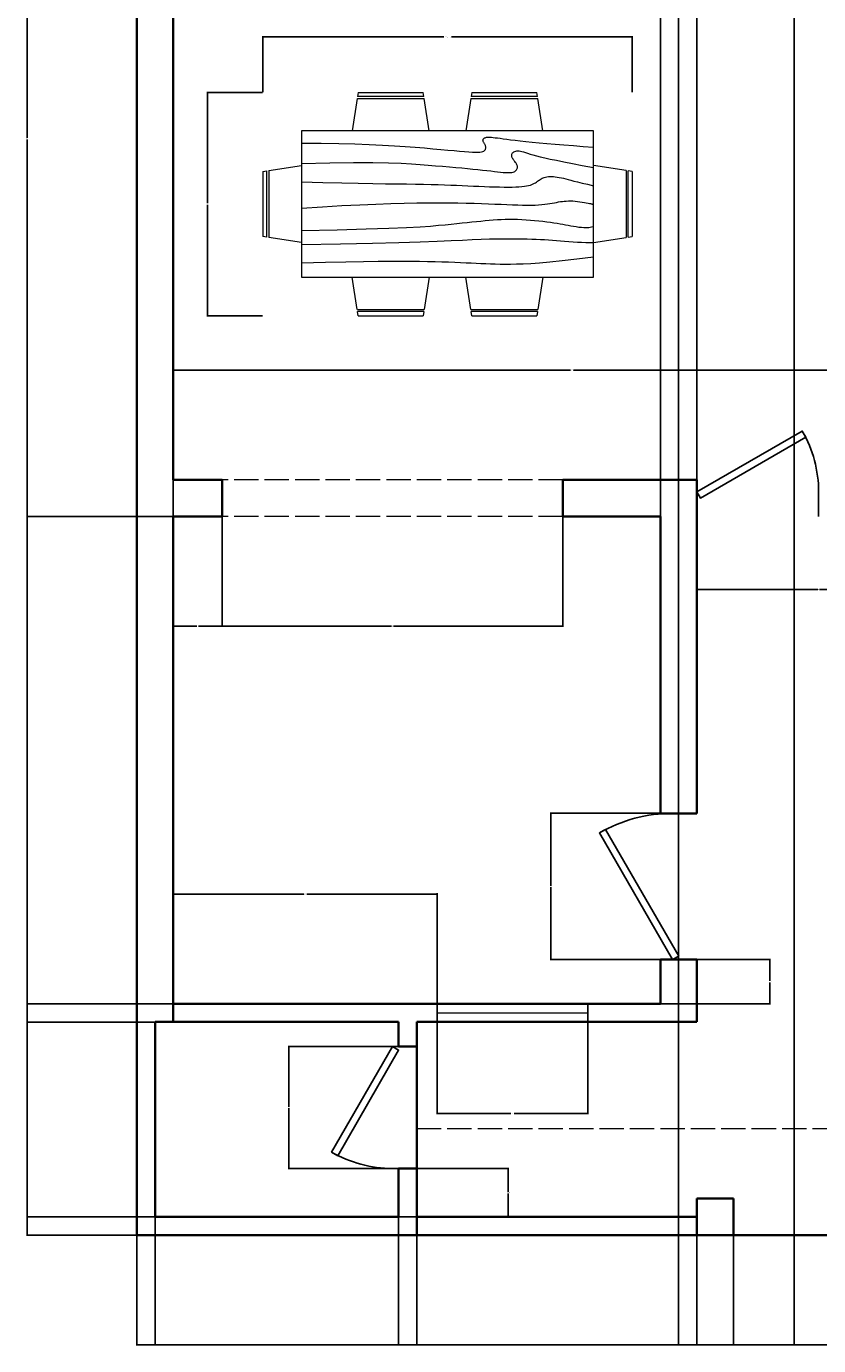
# Model space of a CAD drawing. Units: inches. Extents: x 2599 to 2953, y 557 to 1152.
# Tile 1 of 7: x 2599 to 2794, y 557 to 882. Entities that reach past the tile are written whole.
import ezdxf

# ---------------------------------------------------------------- set-up
doc = ezdxf.new("R2010")
doc.units = ezdxf.units.IN
doc.linetypes.add('ACAD_ISO02W100', pattern=[15, 12, -3])
for name, color, linetype, lineweight in [('A-ANNO-DIMS', 2, 'Continuous', 18), ('A-COLS', 7, 'Continuous', 35), ('A-DOOR', 4, 'Continuous', 25), ('A-FURN', 8, 'Continuous', 18), ('A-GLAZ', 4, 'Continuous', 18), ('A-WALL', 7, 'Continuous', 35), ('A-WALL-OVHD', 8, 'ACAD_ISO02W100', 18)]:
    doc.layers.add(name, color=color, linetype=linetype, lineweight=lineweight)
doc.styles.get("Standard").update_dxf_attribs({"font": 'arial.ttf'})
doc.dimstyles.get("Standard").update_dxf_attribs({"dimtxt": 0.18, "dimasz": 0.18, "dimexe": 0.18, "dimexo": 0.0625, "dimgap": 0.09, "dimtad": 0, "dimtih": 1, "dimtoh": 1, "dimdec": 4, "dimzin": 0, "dimdsep": 46, "dimtxsty": 'Standard', "dimcen": 0.09, "dimadec": 0, "dimazin": 0, "dimtfac": 1, "dimtdec": 4, "dimtofl": 0, "dimtmove": 0, "dimatfit": 3, "dimfxl": 1, "dimtolj": 1, "dimtzin": 0, "dimarcsym": 0})

# ---------------------------------------------------------------- blocks, each defined once
blk = doc.blocks.new('*U3')
for p, q in [((-30, 0), (-30, -6)), ((0, 0), (0, -6))]:
    blk.add_line(p, q)
blk.add_lwpolyline([(0, 0), (-25.98, 15), (-26.86, 13.48), (-0.88, -1.52)], close=True)
blk.add_arc((0, 0), 30, 150, 180)
blk = doc.blocks.new('*U4')
for p, q in [((0, 0), (0, -6)), ((36, 0), (36, -6))]:
    blk.add_line(p, q)
blk.add_lwpolyline([(0, 0), (31.18, 18), (32.05, 16.48), (0.87, -1.52)], close=True)
blk.add_arc((0, 0), 36, 0, 30)
blk = doc.blocks.new('*U5')
for p, q in [((0, 0), (0, -6)), ((30, 0), (30, -6))]:
    blk.add_line(p, q)
blk.add_lwpolyline([(0, 0), (25.98, 15), (26.86, 13.48), (0.87, -1.52)], close=True)
blk.add_arc((0, 0), 30, 0, 30)
blk = doc.blocks.new('Dining Set - 36 x 72 in.')
for p, q in [((-22.2343, 26.00059), (-23.4847, 17.99762)), ((-22.2304, 26), (-5.7608, 26)), ((-22, 27.5), (-22.1562, 26.50042)), ((-5.8416, 26.5), (-22.1534, 26.5)), ((-22, 27.5), (-6, 27.5)), ((-5.8437, 26.49966), (-6, 27.5)), ((-4.5152, 17.99762), (-5.7655, 25.99926)), ((5.7657, 26.00059), (4.5153, 17.99762)), ((5.7696, 26), (22.2392, 26)), ((6, 27.5), (5.8438, 26.50042)), ((22.1584, 26.5), (5.8466, 26.5)), ((6, 27.5), (22, 27.5)), ((22.1563, 26.49966), (22, 27.5)), ((23.4848, 17.99762), (22.2345, 25.99926)), ((36, 18), (-36, 18)), ((-36, 18), (-36, -18)), ((36, -18), (36, 18)), ((-45.5, 8), (-44.5004, 8.15617)), ((-45.5, 8), (-45.5, -8)), ((-44.5, -8.15843), (-44.5, 8.15338)), ((-44.0006, 8.23428), (-35.9976, 9.48474)), ((-44, 8.23041), (-44, -8.23915)), ((44.0006, 8.23428), (35.9976, 9.48474)), ((44, 8.23041), (44, -8.23915)), ((44.5, -8.15843), (44.5, 8.15338)), ((45.5, 8), (44.5005, 8.15617)), ((45.5, 8), (45.5, -8)), ((-44.4997, -8.15631), (-45.5, -8)), ((-35.9976, -9.48476), (-43.9993, -8.2345)), ((35.9976, -9.48476), (43.9993, -8.2345)), ((44.4997, -8.15631), (45.5, -8)), ((-36, -18), (36, -18)), ((-22.2343, -26.0006), (-23.4847, -17.99762)), ((-4.5152, -17.99762), (-5.7655, -25.99928)), ((5.7657, -26.0006), (4.5153, -17.99762)), ((23.4848, -17.99762), (22.2345, -25.99928)), ((-22.2304, -26), (-5.7608, -26)), ((-22, -27.5), (-22.1562, -26.50044)), ((-5.8416, -26.5), (-22.1534, -26.5)), ((-22, -27.5), (-6, -27.5)), ((-5.8437, -26.49967), (-6, -27.5)), ((5.7696, -26), (22.2392, -26)), ((6, -27.5), (5.8438, -26.50044)), ((22.1584, -26.5), (5.8466, -26.5)), ((6, -27.5), (22, -27.5)), ((22.1563, -26.49967), (22, -27.5))]:
    blk.add_line(p, q)
for points in [[(-36, 15), (-31.1772, 14.97754), (-26.8079, 14.91406), (-22.8538, 14.81543), (-19.276, 14.6875), (-16.0362, 14.53613), (-13.0957, 14.36718), (-10.4159, 14.18652), (-7.9583, 14), (-5.6904, 13.81315), (-3.6035, 13.63021), (-1.6954, 13.45508), (0.0365, 13.29166), (1.5945, 13.14388), (2.9811, 13.01562), (4.1988, 12.9108), (5.25, 12.83333), (6.1393, 12.78613), (6.8802, 12.76823), (7.4883, 12.77767), (7.9792, 12.8125), (8.3685, 12.87077), (8.6719, 12.95052), (8.9049, 13.0498), (9.0833, 13.16666), (9.2205, 13.29899), (9.3216, 13.44401), (9.3895, 13.59879), (9.4271, 13.76041), (9.4373, 13.92594), (9.4232, 14.09245), (9.3875, 14.257), (9.3333, 14.41666), (9.2638, 14.56917), (9.1836, 14.71484), (9.0975, 14.85465), (9.0104, 14.98958), (8.9272, 15.1206), (8.8529, 15.2487), (8.7922, 15.37483), (8.75, 15.5), (8.7305, 15.62467), (8.7344, 15.74739), (8.7617, 15.86621), (8.8125, 15.97916), (8.8867, 16.08431), (8.9844, 16.17968), (9.1055, 16.26334), (9.25, 16.33333), (9.4189, 16.38802), (9.6172, 16.42708), (9.8506, 16.45052), (10.125, 16.45833), (10.4463, 16.45052), (10.8203, 16.42708), (11.2529, 16.38802), (11.75, 16.33333), (12.3184, 16.26318), (12.9694, 16.17838), (13.7151, 16.07991), (14.5677, 15.96875), (15.5395, 15.84586), (16.6426, 15.71224), (17.8893, 15.56884), (19.2917, 15.41666), (20.859, 15.25667), (22.5879, 15.08984), (24.4721, 14.91715), (26.5052, 14.73958), (28.6809, 14.5581), (30.9929, 14.3737), (33.4347, 14.18733), (36, 14)], [(-36, 10), (-28.9766, 10.14274), (-23.1725, 10.20442), (-18.4241, 10.19775), (-14.5677, 10.13541), (-11.4399, 10.03011), (-8.877, 9.89453), (-6.7154, 9.74137), (-4.7917, 9.58333), (-2.9698, 9.43082), (-1.2246, 9.28515), (0.4415, 9.14534), (2.026, 9.01041), (3.5266, 8.87939), (4.9408, 8.7513), (6.266, 8.62516), (7.5, 8.5), (8.6411, 8.37549), (9.6914, 8.2539), (10.6538, 8.13818), (11.5312, 8.03125), (12.3267, 7.93603), (13.043, 7.85547), (13.6831, 7.79248), (14.25, 7.75), (14.7471, 7.7303), (15.1797, 7.73307), (15.5537, 7.75732), (15.875, 7.80208), (16.1494, 7.86637), (16.3828, 7.94922), (16.5811, 8.04964), (16.75, 8.16666), (16.8944, 8.29915), (17.0143, 8.44531), (17.1089, 8.60319), (17.1771, 8.77083), (17.218, 8.94629), (17.2305, 9.1276), (17.2137, 9.31282), (17.1667, 9.5), (17.0895, 9.6875), (16.987, 9.875), (16.8649, 10.0625), (16.7292, 10.25), (16.5856, 10.4375), (16.4401, 10.625), (16.2985, 10.8125), (16.1667, 11), (16.05, 11.18733), (15.9518, 11.3737), (15.8752, 11.5581), (15.8229, 11.73958), (15.798, 11.91715), (15.8034, 12.08984), (15.842, 12.25667), (15.9167, 12.41666), (16.0295, 12.56836), (16.1784, 12.70833), (16.3605, 12.83268), (16.5729, 12.9375), (16.8127, 13.01888), (17.0768, 13.07291), (17.3625, 13.0957), (17.6667, 13.08333), (17.9894, 13.03312), (18.3418, 12.94726), (18.7382, 12.82918), (19.1927, 12.68229), (19.7195, 12.51001), (20.3327, 12.31575), (21.0465, 12.10294), (21.875, 11.875), (22.8357, 11.63354), (23.959, 11.37304), (25.2786, 11.08618), (26.8282, 10.76562), (28.6414, 10.40405), (30.752, 9.99414), (33.1936, 9.52856), (36, 9)], [(-36, 5.5), (-30.7157, 5.3348), (-26.069, 5.20963), (-21.9946, 5.11767), (-18.4271, 5.05208), (-15.3009, 5.00602), (-12.5508, 4.97265), (-10.1112, 4.94515), (-7.9167, 4.91666), (-5.909, 4.88167), (-4.0586, 4.83984), (-2.3429, 4.79215), (-0.7396, 4.73958), (0.7739, 4.6831), (2.22, 4.6237), (3.6213, 4.56233), (5, 4.5), (6.373, 4.43782), (7.7344, 4.3776), (9.0723, 4.32129), (10.375, 4.27083), (11.6309, 4.22819), (12.8281, 4.19531), (13.9551, 4.17415), (15, 4.16666), (15.954, 4.17448), (16.819, 4.19791), (17.6001, 4.23698), (18.3021, 4.29166), (18.9299, 4.36198), (19.4883, 4.44791), (19.9823, 4.54948), (20.4167, 4.66666), (20.7969, 4.79899), (21.1302, 4.94401), (21.4245, 5.09879), (21.6875, 5.26041), (21.9271, 5.42594), (22.1511, 5.59245), (22.3672, 5.757), (22.5834, 5.91666), (22.8065, 6.06868), (23.0404, 6.21093), (23.2879, 6.34147), (23.5521, 6.45833), (23.8358, 6.55957), (24.142, 6.64323), (24.4735, 6.70735), (24.8334, 6.75), (25.2235, 6.76969), (25.642, 6.76692), (26.0858, 6.74267), (26.5521, 6.69791), (27.0379, 6.63362), (27.5404, 6.55078), (28.0565, 6.45036), (28.5834, 6.33333), (29.1242, 6.19987), (29.7071, 6.04687), (30.3661, 5.87044), (31.1354, 5.66666), (32.0493, 5.43164), (33.142, 5.16146), (34.4475, 4.85221), (36, 4.5)], [(-36, -1), (-30.7915, -0.6591), (-26.0195, -0.38216), (-21.6519, -0.16284), (-17.6563, 0.00521), (-14.0005, 0.12833), (-10.6523, 0.21289), (-7.5796, 0.26522), (-4.75, 0.29166), (-2.134, 0.29793), (0.2878, 0.28711), (2.5317, 0.26163), (4.6146, 0.22396), (6.5529, 0.17651), (8.3633, 0.12174), (10.0623, 0.06209), (11.6667, 0), (13.1899, -0.06201), (14.6341, -0.1211), (15.9982, -0.17432), (17.2813, -0.21875), (18.4823, -0.25147), (19.6003, -0.26953), (20.6343, -0.27002), (21.5834, -0.25), (22.4481, -0.20768), (23.2357, -0.14584), (23.9549, -0.06836), (24.6146, 0.02083), (25.2235, 0.11784), (25.7904, 0.21875), (26.3241, 0.31966), (26.8334, 0.41666), (27.3265, 0.50618), (27.8099, 0.58593), (28.2894, 0.65397), (28.7709, 0.70833), (29.2601, 0.74707), (29.763, 0.76823), (30.2855, 0.76985), (30.8334, 0.75), (31.4088, 0.70784), (31.9994, 0.64713), (32.589, 0.57275), (33.1615, 0.48958), (33.7008, 0.4025), (34.1908, 0.3164), (34.6153, 0.23616), (34.9584, 0.16666), (35.2099, 0.11165), (35.3848, 0.07031), (35.504, 0.04069), (35.5886, 0.02083), (35.6594, 0.00879), (35.7377, 0.0026), (35.8442, 0.00032), (36, 0)], [(-36, -6.5), (-27.1843, -6.31267), (-20.084, -6.1263), (-14.469, -5.9419), (-10.1094, -5.76042), (-6.7752, -5.58285), (-4.2363, -5.41016), (-2.2629, -5.24333), (-0.625, -5.08334), (0.8708, -4.93099), (2.2715, -4.78646), (3.5872, -4.64974), (4.8281, -4.52084), (6.0046, -4.39974), (7.127, -4.28646), (8.2053, -4.18099), (9.25, -4.08334), (10.2705, -3.99382), (11.2734, -3.91407), (12.2647, -3.84603), (13.25, -3.79167), (14.2354, -3.75293), (15.2266, -3.73177), (16.2295, -3.73015), (17.25, -3.75), (18.2912, -3.79248), (19.3451, -3.85547), (20.4009, -3.93604), (21.4479, -4.03125), (22.4754, -4.13819), (23.4727, -4.25391), (24.4289, -4.37549), (25.3334, -4.5), (26.1785, -4.62492), (26.9694, -4.74935), (27.7145, -4.87281), (28.4219, -4.99479), (29.1, -5.11483), (29.7572, -5.23242), (30.4016, -5.34709), (31.0417, -5.45834), (31.6837, -5.56437), (32.3262, -5.65821), (32.9658, -5.73153), (33.599, -5.77604), (34.2224, -5.78345), (34.8327, -5.74545), (35.4264, -5.65373), (36, -5.5)], [(-36, -10), (-26.4022, -9.81299), (-18.4675, -9.62891), (-11.9839, -9.45069), (-6.7396, -9.28125), (-2.5226, -9.12354), (0.8789, -8.98047), (3.6769, -8.85498), (6.0833, -8.75), (8.2767, -8.66765), (10.3021, -8.60677), (12.1712, -8.56543), (13.8958, -8.54167), (15.4876, -8.53353), (16.9583, -8.53907), (18.3197, -8.55632), (19.5834, -8.58334), (20.7616, -8.61841), (21.8685, -8.66081), (22.9188, -8.71004), (23.9271, -8.76563), (24.9081, -8.82707), (25.8763, -8.89388), (26.8465, -8.96558), (27.8334, -9.04167), (28.8474, -9.12118), (29.8828, -9.20117), (30.93, -9.27824), (31.9792, -9.34896), (33.0205, -9.40991), (34.0443, -9.45768), (35.0407, -9.48885), (36, -9.5)], [(-36, -14.5), (-30.0881, -14.33513), (-25.0332, -14.21224), (-20.7312, -14.12647), (-17.0781, -14.07292), (-13.97, -14.04671), (-11.3027, -14.04297), (-8.9724, -14.05681), (-6.875, -14.08334), (-4.9224, -14.11833), (-3.0905, -14.16016), (-1.3709, -14.20785), (0.2448, -14.26042), (1.7647, -14.3169), (3.1973, -14.3763), (4.5507, -14.43767), (5.8333, -14.5), (7.0554, -14.5621), (8.235, -14.62175), (9.3922, -14.67652), (10.5469, -14.72396), (11.7192, -14.76164), (12.929, -14.78711), (14.1965, -14.79794), (15.5417, -14.79167), (16.9933, -14.76424), (18.6152, -14.70508), (20.4804, -14.60197), (22.6615, -14.44271), (25.2312, -14.21509), (28.2624, -13.9069), (31.8277, -13.50594), (36, -13)]]:
    blk.add_lwpolyline(points)
blk = doc.blocks.new('*D17')
at = {"layer": 'A-ANNO-DIMS', "color": 0, "lineweight": -2, "transparency": 16777216}
for p, q in [((2656.99, 865.8), (2656.99, 879.57)), ((2657.17, 879.39), (2701.54, 879.39)), ((2747.81, 879.39), (2703.44, 879.39)), ((2747.99, 865.8), (2747.99, 879.57))]:
    blk.add_line(p, q, dxfattribs=at)
at = {"layer": 'A-ANNO-DIMS', "color": 0, "transparency": 16777216}
for points in [[(2657.17, 879.42), (2657.17, 879.36), (2656.99, 879.39)], [(2747.81, 879.42), (2747.81, 879.36), (2747.99, 879.39)]]:
    blk.add_solid(points, dxfattribs=at)
at = {"layer": 'Defpoints', "color": 0, "transparency": 16777216}
for p in [(2747.99, 879.39), (2656.99, 865.74), (2747.99, 865.74)]:
    blk.add_point(p, dxfattribs=at)
at = {"layer": 'A-ANNO-DIMS', "color": 0, "transparency": 16777216, "insert": (2702.49, 879.39), "char_height": 0.18, "attachment_point": 5}
blk.add_mtext('\\A1;DINING SET 91', dxfattribs=at)
blk = doc.blocks.new('*D18')
at = {"layer": 'A-ANNO-DIMS', "color": 0, "lineweight": -2, "transparency": 16777216}
for p, q in [((2656.93, 865.74), (2643.16, 865.74)), ((2643.34, 865.56), (2643.34, 838.42)), ((2643.34, 810.92), (2643.34, 838.06)), ((2656.93, 810.74), (2643.16, 810.74))]:
    blk.add_line(p, q, dxfattribs=at)
at = {"layer": 'A-ANNO-DIMS', "color": 0, "transparency": 16777216}
for points in [[(2643.31, 865.56), (2643.37, 865.56), (2643.34, 865.74)], [(2643.31, 810.92), (2643.37, 810.92), (2643.34, 810.74)]]:
    blk.add_solid(points, dxfattribs=at)
at = {"layer": 'Defpoints', "color": 0, "transparency": 16777216}
for p in [(2643.34, 865.74), (2656.99, 865.74), (2656.99, 810.74)]:
    blk.add_point(p, dxfattribs=at)
at = {"layer": 'A-ANNO-DIMS', "color": 0, "transparency": 16777216, "insert": (2643.34, 838.24), "char_height": 0.18, "attachment_point": 5}
blk.add_mtext('\\A1;55', dxfattribs=at)
blk = doc.blocks.new('*D21')
at = {"layer": 'A-ANNO-DIMS', "color": 0, "lineweight": -2, "transparency": 16777216}
for p, q in [((2625.92, 1124.28), (2625.92, 557.16)), ((2925.92, 584.28), (2925.92, 557.16)), ((2626.1, 557.34), (2775.63, 557.34)), ((2925.74, 557.34), (2776.21, 557.34))]:
    blk.add_line(p, q, dxfattribs=at)
at = {"layer": 'A-ANNO-DIMS', "color": 0, "transparency": 16777216}
for points in [[(2626.1, 557.37), (2626.1, 557.31), (2625.92, 557.34)], [(2925.74, 557.37), (2925.74, 557.31), (2925.92, 557.34)]]:
    blk.add_solid(points, dxfattribs=at)
at = {"layer": 'Defpoints', "color": 0, "transparency": 16777216}
for p in [(2625.92, 1124.34), (2925.92, 584.34), (2925.92, 557.34)]:
    blk.add_point(p, dxfattribs=at)
at = {"layer": 'A-ANNO-DIMS', "color": 0, "transparency": 16777216, "insert": (2775.92, 557.34), "char_height": 0.18, "attachment_point": 5}
blk.add_mtext('\\A1;300', dxfattribs=at)
blk = doc.blocks.new('*D22')
at = {"layer": 'A-ANNO-DIMS', "color": 0, "lineweight": -2, "transparency": 16777216}
for p, q in [((2625.86, 1124.34), (2598.74, 1124.34)), ((2598.92, 1124.16), (2598.92, 854.52)), ((2598.92, 584.52), (2598.92, 854.16)), ((2625.86, 584.34), (2598.74, 584.34))]:
    blk.add_line(p, q, dxfattribs=at)
at = {"layer": 'A-ANNO-DIMS', "color": 0, "transparency": 16777216}
for points in [[(2598.89, 1124.16), (2598.95, 1124.16), (2598.92, 1124.34)], [(2598.89, 584.52), (2598.95, 584.52), (2598.92, 584.34)]]:
    blk.add_solid(points, dxfattribs=at)
at = {"layer": 'Defpoints', "color": 0, "transparency": 16777216}
for p in [(2598.92, 1124.34), (2625.92, 1124.34), (2625.92, 584.34)]:
    blk.add_point(p, dxfattribs=at)
at = {"layer": 'A-ANNO-DIMS', "color": 0, "transparency": 16777216, "insert": (2598.92, 854.34), "char_height": 0.18, "attachment_point": 5}
blk.add_mtext('\\A1;540', dxfattribs=at)
blk = doc.blocks.new('*D23')
at = {"layer": 'A-ANNO-DIMS', "color": 0, "lineweight": -2, "transparency": 16777216}
for p, q in [((2634.92, 770.4), (2634.92, 797.53)), ((2635.1, 797.35), (2732.79, 797.35)), ((2831.24, 797.35), (2733.56, 797.35)), ((2831.42, 770.4), (2831.42, 797.53))]:
    blk.add_line(p, q, dxfattribs=at)
at = {"layer": 'A-ANNO-DIMS', "color": 0, "transparency": 16777216}
for points in [[(2635.1, 797.38), (2635.1, 797.32), (2634.92, 797.35)], [(2831.24, 797.38), (2831.24, 797.32), (2831.42, 797.35)]]:
    blk.add_solid(points, dxfattribs=at)
at = {"layer": 'Defpoints', "color": 0, "transparency": 16777216}
for p in [(2831.42, 797.35), (2634.92, 770.34), (2831.42, 770.34)]:
    blk.add_point(p, dxfattribs=at)
at = {"layer": 'A-ANNO-DIMS', "color": 0, "transparency": 16777216, "insert": (2733.17, 797.35), "char_height": 0.18, "attachment_point": 5}
blk.add_mtext('\\A1;196.5', dxfattribs=at)
blk = doc.blocks.new('*D28')
at = {"layer": 'A-ANNO-DIMS', "color": 0, "lineweight": -2, "transparency": 16777216}
for p, q in [((2763.92, 770.28), (2763.92, 743.16)), ((2823.92, 770.28), (2823.92, 743.16)), ((2764.1, 743.34), (2793.7, 743.34)), ((2823.74, 743.34), (2794.14, 743.34))]:
    blk.add_line(p, q, dxfattribs=at)
at = {"layer": 'A-ANNO-DIMS', "color": 0, "transparency": 16777216}
for points in [[(2764.1, 743.37), (2764.1, 743.31), (2763.92, 743.34)], [(2823.74, 743.37), (2823.74, 743.31), (2823.92, 743.34)]]:
    blk.add_solid(points, dxfattribs=at)
at = {"layer": 'Defpoints', "color": 0, "transparency": 16777216}
for p in [(2763.92, 770.34), (2823.92, 770.34), (2763.92, 743.34)]:
    blk.add_point(p, dxfattribs=at)
at = {"layer": 'A-ANNO-DIMS', "color": 0, "transparency": 16777216, "insert": (2793.92, 743.34), "char_height": 0.18, "attachment_point": 5}
blk.add_mtext('\\A1;60', dxfattribs=at)
blk = doc.blocks.new('*D32')
at = {"layer": 'A-ANNO-DIMS', "color": 0, "lineweight": -2, "transparency": 16777216}
for p, q in [((2630.42, 588.78), (2630.42, 557.16)), ((2690.42, 588.78), (2690.42, 557.16)), ((2630.6, 557.34), (2660.2, 557.34)), ((2690.24, 557.34), (2660.64, 557.34))]:
    blk.add_line(p, q, dxfattribs=at)
at = {"layer": 'A-ANNO-DIMS', "color": 0, "transparency": 16777216}
for points in [[(2630.6, 557.37), (2630.6, 557.31), (2630.42, 557.34)], [(2690.24, 557.37), (2690.24, 557.31), (2690.42, 557.34)]]:
    blk.add_solid(points, dxfattribs=at)
at = {"layer": 'Defpoints', "color": 0, "transparency": 16777216}
for p in [(2630.42, 588.84), (2690.42, 588.84), (2690.42, 557.34)]:
    blk.add_point(p, dxfattribs=at)
at = {"layer": 'A-ANNO-DIMS', "color": 0, "transparency": 16777216, "insert": (2660.42, 557.34), "char_height": 0.18, "attachment_point": 5}
blk.add_mtext('\\A1;60', dxfattribs=at)
blk = doc.blocks.new('*D33')
at = {"layer": 'A-ANNO-DIMS', "color": 0, "lineweight": -2, "transparency": 16777216}
for p, q in [((2630.36, 636.84), (2598.74, 636.84)), ((2598.92, 636.66), (2598.92, 613.02)), ((2598.92, 589.02), (2598.92, 612.66)), ((2630.36, 588.84), (2598.74, 588.84))]:
    blk.add_line(p, q, dxfattribs=at)
at = {"layer": 'A-ANNO-DIMS', "color": 0, "transparency": 16777216}
for points in [[(2598.89, 636.66), (2598.95, 636.66), (2598.92, 636.84)], [(2598.89, 589.02), (2598.95, 589.02), (2598.92, 588.84)]]:
    blk.add_solid(points, dxfattribs=at)
at = {"layer": 'Defpoints', "color": 0, "transparency": 16777216}
for p in [(2598.92, 636.84), (2630.42, 636.84), (2630.42, 588.84)]:
    blk.add_point(p, dxfattribs=at)
at = {"layer": 'A-ANNO-DIMS', "color": 0, "transparency": 16777216, "insert": (2598.92, 612.84), "char_height": 0.18, "attachment_point": 5}
blk.add_mtext('\\A1;48', dxfattribs=at)
blk = doc.blocks.new('*D34')
at = {"layer": 'A-ANNO-DIMS', "color": 0, "lineweight": -2, "transparency": 16777216}
for p, q in [((2694.92, 584.28), (2694.92, 557.16)), ((2763.92, 584.28), (2763.92, 557.16)), ((2695.1, 557.34), (2729.2, 557.34)), ((2763.74, 557.34), (2729.64, 557.34))]:
    blk.add_line(p, q, dxfattribs=at)
at = {"layer": 'A-ANNO-DIMS', "color": 0, "transparency": 16777216}
for points in [[(2695.1, 557.37), (2695.1, 557.31), (2694.92, 557.34)], [(2763.74, 557.37), (2763.74, 557.31), (2763.92, 557.34)]]:
    blk.add_solid(points, dxfattribs=at)
at = {"layer": 'Defpoints', "color": 0, "transparency": 16777216}
for p in [(2694.92, 584.34), (2763.92, 584.34), (2763.92, 557.34)]:
    blk.add_point(p, dxfattribs=at)
at = {"layer": 'A-ANNO-DIMS', "color": 0, "transparency": 16777216, "insert": (2729.42, 557.34), "char_height": 0.18, "attachment_point": 5}
blk.add_mtext('\\A1;69', dxfattribs=at)
blk = doc.blocks.new('*D35')
at = {"layer": 'A-ANNO-DIMS', "color": 0, "lineweight": -2, "transparency": 16777216}
for p, q in [((2763.92, 584.28), (2763.92, 557.16)), ((2772.92, 584.28), (2772.92, 557.16)), ((2764.1, 557.34), (2768.27, 557.34)), ((2772.74, 557.34), (2768.57, 557.34))]:
    blk.add_line(p, q, dxfattribs=at)
at = {"layer": 'A-ANNO-DIMS', "color": 0, "transparency": 16777216}
for points in [[(2764.1, 557.37), (2764.1, 557.31), (2763.92, 557.34)], [(2772.74, 557.37), (2772.74, 557.31), (2772.92, 557.34)]]:
    blk.add_solid(points, dxfattribs=at)
at = {"layer": 'Defpoints', "color": 0, "transparency": 16777216}
for p in [(2763.92, 584.34), (2772.92, 584.34), (2772.92, 557.34)]:
    blk.add_point(p, dxfattribs=at)
at = {"layer": 'A-ANNO-DIMS', "color": 0, "transparency": 16777216, "insert": (2768.42, 557.34), "char_height": 0.18, "attachment_point": 5}
blk.add_mtext('\\A1;9', dxfattribs=at)
blk = doc.blocks.new('*D36')
at = {"layer": 'A-ANNO-DIMS', "color": 0, "lineweight": -2, "transparency": 16777216}
for p, q in [((2772.92, 584.28), (2772.92, 557.16)), ((2916.92, 584.28), (2916.92, 557.16)), ((2773.1, 557.34), (2844.64, 557.34)), ((2916.74, 557.34), (2845.2, 557.34))]:
    blk.add_line(p, q, dxfattribs=at)
at = {"layer": 'A-ANNO-DIMS', "color": 0, "transparency": 16777216}
for points in [[(2773.1, 557.37), (2773.1, 557.31), (2772.92, 557.34)], [(2916.74, 557.37), (2916.74, 557.31), (2916.92, 557.34)]]:
    blk.add_solid(points, dxfattribs=at)
at = {"layer": 'Defpoints', "color": 0, "transparency": 16777216}
for p in [(2772.92, 584.34), (2916.92, 584.34), (2916.92, 557.34)]:
    blk.add_point(p, dxfattribs=at)
at = {"layer": 'A-ANNO-DIMS', "color": 0, "transparency": 16777216, "insert": (2844.92, 557.34), "char_height": 0.18, "attachment_point": 5}
blk.add_mtext('\\A1;144', dxfattribs=at)
blk = doc.blocks.new('*D37')
at = {"layer": 'A-ANNO-DIMS', "color": 0, "lineweight": -2, "transparency": 16777216}
for p, q in [((2634.92, 761.4), (2634.92, 1151.53)), ((2635.1, 1151.35), (2694.64, 1151.35)), ((2754.74, 1151.35), (2695.2, 1151.35)), ((2754.92, 761.4), (2754.92, 1151.53))]:
    blk.add_line(p, q, dxfattribs=at)
at = {"layer": 'A-ANNO-DIMS', "color": 0, "transparency": 16777216}
for points in [[(2635.1, 1151.38), (2635.1, 1151.32), (2634.92, 1151.35)], [(2754.74, 1151.38), (2754.74, 1151.32), (2754.92, 1151.35)]]:
    blk.add_solid(points, dxfattribs=at)
at = {"layer": 'Defpoints', "color": 0, "transparency": 16777216}
for p in [(2754.92, 1151.35), (2634.92, 761.34), (2754.92, 761.34)]:
    blk.add_point(p, dxfattribs=at)
at = {"layer": 'A-ANNO-DIMS', "color": 0, "transparency": 16777216, "insert": (2694.92, 1151.35), "char_height": 0.18, "attachment_point": 5}
blk.add_mtext('\\A1;120', dxfattribs=at)
blk = doc.blocks.new('*D38')
at = {"layer": 'A-ANNO-DIMS', "color": 0, "lineweight": -2, "transparency": 16777216}
for p, q in [((2763.92, 761.4), (2763.92, 1151.53)), ((2764.1, 1151.35), (2821.14, 1151.35)), ((2878.74, 1151.35), (2821.7, 1151.35)), ((2878.92, 761.4), (2878.92, 1151.53))]:
    blk.add_line(p, q, dxfattribs=at)
at = {"layer": 'A-ANNO-DIMS', "color": 0, "transparency": 16777216}
for points in [[(2764.1, 1151.38), (2764.1, 1151.32), (2763.92, 1151.35)], [(2878.74, 1151.38), (2878.74, 1151.32), (2878.92, 1151.35)]]:
    blk.add_solid(points, dxfattribs=at)
at = {"layer": 'Defpoints', "color": 0, "transparency": 16777216}
for p in [(2878.92, 1151.35), (2763.92, 761.34), (2878.92, 761.34)]:
    blk.add_point(p, dxfattribs=at)
at = {"layer": 'A-ANNO-DIMS', "color": 0, "transparency": 16777216, "insert": (2821.42, 1151.35), "char_height": 0.18, "attachment_point": 5}
blk.add_mtext('\\A1;115', dxfattribs=at)
blk = doc.blocks.new('*D45')
at = {"layer": 'A-ANNO-DIMS', "color": 0, "lineweight": -2, "transparency": 16777216}
for p, q in [((2634.86, 761.34), (2598.74, 761.34)), ((2598.92, 761.16), (2598.92, 701.52)), ((2598.92, 641.52), (2598.92, 701.16)), ((2634.86, 641.34), (2598.74, 641.34))]:
    blk.add_line(p, q, dxfattribs=at)
at = {"layer": 'A-ANNO-DIMS', "color": 0, "transparency": 16777216}
for points in [[(2598.89, 761.16), (2598.95, 761.16), (2598.92, 761.34)], [(2598.89, 641.52), (2598.95, 641.52), (2598.92, 641.34)]]:
    blk.add_solid(points, dxfattribs=at)
at = {"layer": 'Defpoints', "color": 0, "transparency": 16777216}
for p in [(2598.92, 761.34), (2634.92, 761.34), (2634.92, 641.34)]:
    blk.add_point(p, dxfattribs=at)
at = {"layer": 'A-ANNO-DIMS', "color": 0, "transparency": 16777216, "insert": (2598.92, 701.34), "char_height": 0.18, "attachment_point": 5}
blk.add_mtext('\\A1;120', dxfattribs=at)
blk = doc.blocks.new('*D46')
at = {"layer": 'A-ANNO-DIMS', "color": 0, "lineweight": -2, "transparency": 16777216}
for p, q in [((2754.86, 688.22), (2727.74, 688.22)), ((2727.92, 688.04), (2727.92, 670.4)), ((2727.92, 652.4), (2727.92, 670.04)), ((2754.86, 652.22), (2727.74, 652.22))]:
    blk.add_line(p, q, dxfattribs=at)
at = {"layer": 'A-ANNO-DIMS', "color": 0, "transparency": 16777216}
for points in [[(2727.89, 688.04), (2727.95, 688.04), (2727.92, 688.22)], [(2727.89, 652.4), (2727.95, 652.4), (2727.92, 652.22)]]:
    blk.add_solid(points, dxfattribs=at)
at = {"layer": 'Defpoints', "color": 0, "transparency": 16777216}
for p in [(2727.92, 688.22), (2754.92, 688.22), (2754.92, 652.22)]:
    blk.add_point(p, dxfattribs=at)
at = {"layer": 'A-ANNO-DIMS', "color": 0, "transparency": 16777216, "insert": (2727.92, 670.22), "char_height": 0.18, "attachment_point": 5}
blk.add_mtext('\\A1;36', dxfattribs=at)
blk = doc.blocks.new('*D47')
at = {"layer": 'A-ANNO-DIMS', "color": 0, "lineweight": -2, "transparency": 16777216}
for p, q in [((2754.98, 652.22), (2782.1, 652.22)), ((2781.92, 652.04), (2781.92, 646.96)), ((2781.92, 641.52), (2781.92, 646.6)), ((2754.98, 641.34), (2782.1, 641.34))]:
    blk.add_line(p, q, dxfattribs=at)
at = {"layer": 'A-ANNO-DIMS', "color": 0, "transparency": 16777216}
for points in [[(2781.89, 652.04), (2781.95, 652.04), (2781.92, 652.22)], [(2781.89, 641.52), (2781.95, 641.52), (2781.92, 641.34)]]:
    blk.add_solid(points, dxfattribs=at)
at = {"layer": 'Defpoints', "color": 0, "transparency": 16777216}
for p in [(2754.92, 652.22), (2754.92, 641.34), (2781.92, 641.34)]:
    blk.add_point(p, dxfattribs=at)
at = {"layer": 'A-ANNO-DIMS', "color": 0, "transparency": 16777216, "insert": (2781.92, 646.78), "char_height": 0.18, "attachment_point": 5}
blk.add_mtext('\\A1;10.877', dxfattribs=at)
blk = doc.blocks.new('*D48')
at = {"layer": 'A-ANNO-DIMS', "color": 0, "lineweight": -2, "transparency": 16777216}
for p, q in [((2634.92, 761.28), (2634.92, 734.16)), ((2646.92, 761.28), (2646.92, 734.16)), ((2635.1, 734.34), (2640.71, 734.34)), ((2646.74, 734.34), (2641.13, 734.34))]:
    blk.add_line(p, q, dxfattribs=at)
at = {"layer": 'A-ANNO-DIMS', "color": 0, "transparency": 16777216}
for points in [[(2635.1, 734.37), (2635.1, 734.31), (2634.92, 734.34)], [(2646.74, 734.37), (2646.74, 734.31), (2646.92, 734.34)]]:
    blk.add_solid(points, dxfattribs=at)
at = {"layer": 'Defpoints', "color": 0, "transparency": 16777216}
for p in [(2634.92, 761.34), (2646.92, 761.34), (2634.92, 734.34)]:
    blk.add_point(p, dxfattribs=at)
at = {"layer": 'A-ANNO-DIMS', "color": 0, "transparency": 16777216, "insert": (2640.92, 734.34), "char_height": 0.18, "attachment_point": 5}
blk.add_mtext('\\A1;12', dxfattribs=at)
blk = doc.blocks.new('*D49')
at = {"layer": 'A-ANNO-DIMS', "color": 0, "lineweight": -2, "transparency": 16777216}
for p, q in [((2646.92, 761.28), (2646.92, 734.16)), ((2730.92, 761.28), (2730.92, 734.16)), ((2647.1, 734.34), (2688.7, 734.34)), ((2730.74, 734.34), (2689.14, 734.34))]:
    blk.add_line(p, q, dxfattribs=at)
at = {"layer": 'A-ANNO-DIMS', "color": 0, "transparency": 16777216}
for points in [[(2647.1, 734.37), (2647.1, 734.31), (2646.92, 734.34)], [(2730.74, 734.37), (2730.74, 734.31), (2730.92, 734.34)]]:
    blk.add_solid(points, dxfattribs=at)
at = {"layer": 'Defpoints', "color": 0, "transparency": 16777216}
for p in [(2646.92, 761.34), (2730.92, 761.34), (2646.92, 734.34)]:
    blk.add_point(p, dxfattribs=at)
at = {"layer": 'A-ANNO-DIMS', "color": 0, "transparency": 16777216, "insert": (2688.92, 734.34), "char_height": 0.18, "attachment_point": 5}
blk.add_mtext('\\A1;84', dxfattribs=at)
blk = doc.blocks.new('*D50')
at = {"layer": 'A-ANNO-DIMS', "color": 0, "lineweight": -2, "transparency": 16777216}
for p, q in [((2699.95, 641.28), (2699.95, 614.16)), ((2737.03, 641.28), (2737.03, 614.16)), ((2700.13, 614.34), (2718.1, 614.34)), ((2736.85, 614.34), (2718.89, 614.34))]:
    blk.add_line(p, q, dxfattribs=at)
at = {"layer": 'A-ANNO-DIMS', "color": 0, "transparency": 16777216}
for points in [[(2700.13, 614.37), (2700.13, 614.31), (2699.95, 614.34)], [(2736.85, 614.37), (2736.85, 614.31), (2737.03, 614.34)]]:
    blk.add_solid(points, dxfattribs=at)
at = {"layer": 'Defpoints', "color": 0, "transparency": 16777216}
for p in [(2699.95, 641.34), (2737.03, 641.34), (2699.95, 614.34)]:
    blk.add_point(p, dxfattribs=at)
at = {"layer": 'A-ANNO-DIMS', "color": 0, "transparency": 16777216, "insert": (2718.49, 614.34), "char_height": 0.18, "attachment_point": 5}
blk.add_mtext('\\A1;37.08', dxfattribs=at)
blk = doc.blocks.new('*D51')
at = {"layer": 'A-ANNO-DIMS', "color": 0, "lineweight": -2, "transparency": 16777216}
for p, q in [((2634.92, 641.4), (2634.92, 668.53)), ((2635.1, 668.35), (2667.04, 668.35)), ((2699.77, 668.35), (2667.83, 668.35)), ((2699.95, 641.4), (2699.95, 668.53))]:
    blk.add_line(p, q, dxfattribs=at)
at = {"layer": 'A-ANNO-DIMS', "color": 0, "transparency": 16777216}
for points in [[(2635.1, 668.38), (2635.1, 668.32), (2634.92, 668.35)], [(2699.77, 668.38), (2699.77, 668.32), (2699.95, 668.35)]]:
    blk.add_solid(points, dxfattribs=at)
at = {"layer": 'Defpoints', "color": 0, "transparency": 16777216}
for p in [(2699.95, 668.35), (2634.92, 641.34), (2699.95, 641.34)]:
    blk.add_point(p, dxfattribs=at)
at = {"layer": 'A-ANNO-DIMS', "color": 0, "transparency": 16777216, "insert": (2667.44, 668.35), "char_height": 0.18, "attachment_point": 5}
blk.add_mtext('\\A1;65.03', dxfattribs=at)
blk = doc.blocks.new('*D52')
at = {"layer": 'A-ANNO-DIMS', "color": 0, "lineweight": -2, "transparency": 16777216}
for p, q in [((2690.36, 630.79), (2663.24, 630.79)), ((2663.42, 630.61), (2663.42, 615.97)), ((2663.42, 600.97), (2663.42, 615.6)), ((2690.36, 600.79), (2663.24, 600.79))]:
    blk.add_line(p, q, dxfattribs=at)
at = {"layer": 'A-ANNO-DIMS', "color": 0, "transparency": 16777216}
for points in [[(2663.39, 630.61), (2663.45, 630.61), (2663.42, 630.79)], [(2663.39, 600.97), (2663.45, 600.97), (2663.42, 600.79)]]:
    blk.add_solid(points, dxfattribs=at)
at = {"layer": 'Defpoints', "color": 0, "transparency": 16777216}
for p in [(2663.42, 630.79), (2690.42, 630.79), (2690.42, 600.79)]:
    blk.add_point(p, dxfattribs=at)
at = {"layer": 'A-ANNO-DIMS', "color": 0, "transparency": 16777216, "insert": (2663.42, 615.79), "char_height": 0.18, "attachment_point": 5}
blk.add_mtext('\\A1;30', dxfattribs=at)
blk = doc.blocks.new('*D53')
at = {"layer": 'A-ANNO-DIMS', "color": 0, "lineweight": -2, "transparency": 16777216}
for p, q in [((2690.48, 600.79), (2717.6, 600.79)), ((2717.42, 600.61), (2717.42, 595)), ((2717.42, 589.02), (2717.42, 594.63)), ((2690.48, 588.84), (2717.6, 588.84))]:
    blk.add_line(p, q, dxfattribs=at)
at = {"layer": 'A-ANNO-DIMS', "color": 0, "transparency": 16777216}
for points in [[(2717.39, 600.61), (2717.45, 600.61), (2717.42, 600.79)], [(2717.39, 589.02), (2717.45, 589.02), (2717.42, 588.84)]]:
    blk.add_solid(points, dxfattribs=at)
at = {"layer": 'Defpoints', "color": 0, "transparency": 16777216}
for p in [(2690.42, 600.79), (2690.42, 588.84), (2717.42, 588.84)]:
    blk.add_point(p, dxfattribs=at)
at = {"layer": 'A-ANNO-DIMS', "color": 0, "transparency": 16777216, "insert": (2717.42, 594.81), "char_height": 0.18, "attachment_point": 5}
blk.add_mtext('\\A1;11.944', dxfattribs=at)
blk = doc.blocks.new('*D55')
at = {"layer": 'A-ANNO-DIMS', "color": 0, "lineweight": -2, "transparency": 16777216}
for p, q in [((2759.42, 911.28), (2759.42, 557.16)), ((2787.92, 911.28), (2787.92, 557.16)), ((2759.6, 557.34), (2773.35, 557.34)), ((2787.74, 557.34), (2774, 557.34))]:
    blk.add_line(p, q, dxfattribs=at)
at = {"layer": 'A-ANNO-DIMS', "color": 0, "transparency": 16777216}
for points in [[(2759.6, 557.37), (2759.6, 557.31), (2759.42, 557.34)], [(2787.74, 557.37), (2787.74, 557.31), (2787.92, 557.34)]]:
    blk.add_solid(points, dxfattribs=at)
at = {"layer": 'Defpoints', "color": 0, "transparency": 16777216}
for p in [(2759.42, 911.34), (2787.92, 911.34), (2787.92, 557.34)]:
    blk.add_point(p, dxfattribs=at)
at = {"layer": 'A-ANNO-DIMS', "color": 0, "transparency": 16777216, "insert": (2773.67, 557.34), "char_height": 0.18, "attachment_point": 5}
blk.add_mtext('\\A1;28.5', dxfattribs=at)

msp = doc.modelspace()

# ---------------------------------------------------------------- linework, layer by layer
at = {"layer": 'A-COLS'}
for p, q in [((2763.9211, 584.3417), (2763.9211, 593.3417)), ((2763.9211, 593.3417), (2772.9211, 593.3417)), ((2772.9211, 593.3417), (2772.9211, 584.3417))]:
    msp.add_line(p, q, dxfattribs=at)
at = {"layer": 'A-GLAZ'}
for p, q in [((2699.9522, 636.8417), (2699.9522, 641.3417)), ((2737.0325, 641.3417), (2737.0325, 636.8417)), ((2699.9522, 639.0917), (2737.0325, 639.0917))]:
    msp.add_line(p, q, dxfattribs=at)
at = {"layer": 'A-WALL'}
for p, q in [((2625.9211, 1124.3417), (2625.9211, 584.3417)), ((2634.9211, 902.3417), (2634.9211, 770.3417)), ((2646.9211, 770.3417), (2634.9211, 770.3417)), ((2646.9211, 761.3417), (2646.9211, 770.3417)), ((2763.9211, 770.3417), (2730.9211, 770.3417)), ((2730.9211, 761.3417), (2730.9211, 770.3417)), ((2763.9211, 688.2187), (2763.9211, 770.3417)), ((2634.9211, 761.3417), (2634.9211, 636.8417)), ((2646.9211, 761.3417), (2634.9211, 761.3417)), ((2754.9211, 761.3417), (2730.9211, 761.3417)), ((2754.9211, 688.2187), (2754.9211, 761.3417)), ((2754.9211, 688.2187), (2763.9211, 688.2187)), ((2754.9211, 641.3417), (2754.9211, 652.2187)), ((2754.9211, 652.2187), (2763.9211, 652.2187)), ((2763.9211, 636.8417), (2763.9211, 652.2187)), ((2634.9211, 641.3417), (2754.9211, 641.3417)), ((2630.4211, 588.8417), (2630.4211, 636.8417)), ((2630.4211, 636.8417), (2690.4211, 636.8417)), ((2690.4211, 636.8417), (2690.4211, 630.786)), ((2694.9211, 636.8417), (2694.9211, 584.3417)), ((2694.9211, 636.8417), (2763.9211, 636.8417)), ((2690.4211, 630.786), (2694.9211, 630.786)), ((2690.4211, 600.786), (2694.9211, 600.786)), ((2690.4211, 600.786), (2690.4211, 588.8417)), ((2630.4211, 588.8417), (2690.4211, 588.8417)), ((2694.9211, 588.8417), (2763.9211, 588.8417)), ((2625.9211, 584.3417), (2925.9211, 584.3417))]:
    msp.add_line(p, q, dxfattribs=at)
at = {"layer": 'A-WALL-OVHD', "ltscale": 0.5}
for p, q in [((2730.9211, 770.3417), (2646.9211, 770.3417)), ((2730.9211, 761.3417), (2646.9211, 761.3417)), ((2694.9211, 610.5917), (2916.9211, 610.5917))]:
    msp.add_line(p, q, dxfattribs=at)

# ---------------------------------------------------------------- block references
at = {"layer": 'A-DOOR'}
msp.add_blockref('*U5', (2763.9211, 767.3417), dxfattribs=at)
at = {"layer": 'A-DOOR', "rotation": 90}
for name, p in [('*U4', (2757.9211, 652.2187)), ('*U3', (2688.9211, 630.786))]:
    msp.add_blockref(name, p, dxfattribs=at)
at = {"layer": 'A-FURN'}
msp.add_blockref('Dining Set - 36 x 72 in.', (2702.4919, 838.2423), dxfattribs=at)

# ---------------------------------------------------------------- dimensions: what is measured, and where the dimension line sits
at = {"layer": 'A-ANNO-DIMS'}
for base, p1, p2, override, picture, middle in [((2754.9211, 1151.3452), (2634.9211, 761.3417), (2754.9211, 761.3417), {"dimdec": 0, "dimlfac": 1, "dimrnd": 0, "dimzin": 0, "dimdsep": 46, "dimlunit": 2}, '*D37', (2694.9211, 1151.3452)), ((2878.9211, 1151.3452), (2763.9211, 761.3417), (2878.9211, 761.3417), {"dimdec": 0, "dimlfac": 1, "dimrnd": 0, "dimzin": 0, "dimdsep": 46, "dimlunit": 2}, '*D38', (2821.4211, 1151.3452)), ((2925.9211, 557.3382), (2625.9211, 1124.3417), (2925.9211, 584.3417), {"dimdec": 0, "dimlfac": 1, "dimrnd": 0, "dimzin": 0, "dimdsep": 46, "dimlunit": 2}, '*D21', (2775.9211, 557.3382)), ((2787.9211, 557.3382), (2759.4211, 911.3417), (2787.9211, 911.3417), {"dimdec": 1, "dimlfac": 1, "dimrnd": 0, "dimzin": 0, "dimdsep": 46, "dimlunit": 2}, '*D55', (2773.6711, 557.3382)), ((2831.4243, 797.3452), (2634.9211, 770.3417), (2831.4243, 770.3417), {"dimdec": 1, "dimlfac": 1, "dimrnd": 0, "dimzin": 0, "dimdsep": 46, "dimlunit": 2}, '*D23', (2733.1727, 797.3452)), ((2699.9522, 668.3452), (2634.9211, 641.3417), (2699.9522, 641.3417), {"dimdec": 2, "dimlfac": 1, "dimrnd": 0, "dimzin": 0, "dimdsep": 46, "dimlunit": 2}, '*D51', (2667.4367, 668.3452)), ((2690.4211, 557.3382), (2630.4211, 588.8417), (2690.4211, 588.8417), {"dimdec": 0, "dimlfac": 1, "dimrnd": 0, "dimzin": 0, "dimdsep": 46, "dimlunit": 2}, '*D32', (2660.4211, 557.3382)), ((2763.9211, 557.3382), (2694.9211, 584.3417), (2763.9211, 584.3417), {"dimdec": 0, "dimlfac": 1, "dimrnd": 0, "dimzin": 0, "dimdsep": 46, "dimlunit": 2}, '*D34', (2729.4211, 557.3382)), ((2772.9211, 557.3382), (2763.9211, 584.3417), (2772.9211, 584.3417), {"dimdec": 0, "dimlfac": 1, "dimrnd": 0, "dimzin": 0, "dimdsep": 46, "dimlunit": 2}, '*D35', (2768.4211, 557.3382)), ((2916.9211, 557.3382), (2772.9211, 584.3417), (2916.9211, 584.3417), {"dimdec": 0, "dimlfac": 1, "dimrnd": 0, "dimzin": 0, "dimdsep": 46, "dimlunit": 2}, '*D36', (2844.9211, 557.3382))]:
    dim = msp.add_linear_dim(base=base, p1=p1, p2=p2, dimstyle='Standard', override=override, dxfattribs=at)
    dim.commit()
    dim.dimension.update_dxf_attribs({"geometry": picture, "text_midpoint": middle})
for base, p1, p2, angle, override, picture, middle in [((2598.9176, 1124.3417), (2625.9211, 584.3417), (2625.9211, 1124.3417), 90, {"dimdec": 0, "dimlfac": 1, "dimrnd": 0, "dimzin": 0, "dimdsep": 46, "dimlunit": 2}, '*D22', (2598.9176, 854.3417)), ((2643.3419, 865.7423), (2656.9919, 810.7423), (2656.9919, 865.7423), 90, {"dimdec": 0, "dimlfac": 1, "dimrnd": 0, "dimzin": 0, "dimdsep": 46, "dimlunit": 2}, '*D18', (2643.3419, 838.2423)), ((2763.9211, 743.3382), (2823.9243, 770.3417), (2763.9211, 770.3417), 180, {"dimdec": 0, "dimlfac": 1, "dimrnd": 0, "dimzin": 0, "dimdsep": 46, "dimlunit": 2}, '*D28', (2793.9227, 743.3382)), ((2598.9176, 761.3417), (2634.9211, 641.3417), (2634.9211, 761.3417), 90, {"dimdec": 0, "dimlfac": 1, "dimrnd": 0, "dimzin": 0, "dimdsep": 46, "dimlunit": 2}, '*D45', (2598.9176, 701.3417)), ((2634.9211, 734.3382), (2646.9211, 761.3417), (2634.9211, 761.3417), 180, {"dimdec": 0, "dimlfac": 1, "dimrnd": 0, "dimzin": 0, "dimdsep": 46, "dimlunit": 2}, '*D48', (2640.9211, 734.3382)), ((2646.9211, 734.3382), (2730.9211, 761.3417), (2646.9211, 761.3417), 180, {"dimdec": 0, "dimlfac": 1, "dimrnd": 0, "dimzin": 0, "dimdsep": 46, "dimlunit": 2}, '*D49', (2688.9211, 734.3382)), ((2727.9176, 688.2187), (2754.9211, 652.2187), (2754.9211, 688.2187), 90, {"dimdec": 0, "dimlfac": 1, "dimrnd": 0, "dimzin": 0, "dimdsep": 46, "dimlunit": 2}, '*D46', (2727.9176, 670.2187)), ((2781.9246, 641.3417), (2754.9211, 652.2187), (2754.9211, 641.3417), 270, {"dimdec": 3, "dimlfac": 1, "dimrnd": 0, "dimzin": 0, "dimdsep": 46, "dimlunit": 2}, '*D47', (2781.9246, 646.7802)), ((2699.9522, 614.3382), (2737.0325, 641.3417), (2699.9522, 641.3417), 180, {"dimdec": 2, "dimlfac": 1, "dimrnd": 0, "dimzin": 0, "dimdsep": 46, "dimlunit": 2}, '*D50', (2718.4924, 614.3382)), ((2598.9176, 636.8417), (2630.4211, 588.8417), (2630.4211, 636.8417), 90, {"dimdec": 0, "dimlfac": 1, "dimrnd": 0, "dimzin": 0, "dimdsep": 46, "dimlunit": 2}, '*D33', (2598.9176, 612.8417)), ((2663.4176, 630.786), (2690.4211, 600.786), (2690.4211, 630.786), 90, {"dimdec": 0, "dimlfac": 1, "dimrnd": 0, "dimzin": 0, "dimdsep": 46, "dimlunit": 2}, '*D52', (2663.4176, 615.786)), ((2717.4246, 588.8417), (2690.4211, 600.786), (2690.4211, 588.8417), 270, {"dimdec": 3, "dimlfac": 1, "dimrnd": 0, "dimzin": 0, "dimdsep": 46, "dimlunit": 2}, '*D53', (2717.4246, 594.8138))]:
    dim = msp.add_linear_dim(base=base, p1=p1, p2=p2, angle=angle, dimstyle='Standard', override=override, dxfattribs=at)
    dim.commit()
    dim.dimension.update_dxf_attribs({"geometry": picture, "text_midpoint": middle})
dim = msp.add_linear_dim(base=(2747.9919, 879.3923), p1=(2656.9919, 865.7423), p2=(2747.9919, 865.7423), text='DINING SET <>', dimstyle='Standard', override={"dimdec": 0, "dimlfac": 1, "dimrnd": 0, "dimzin": 0, "dimdsep": 46, "dimlunit": 2}, dxfattribs=at)
dim.commit()
dim.dimension.update_dxf_attribs({"geometry": '*D17', "text_midpoint": (2702.4919, 879.3923)})

doc.saveas('drawing.dxf')
